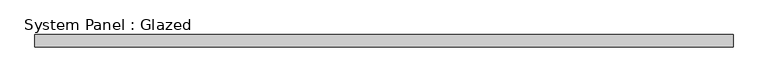
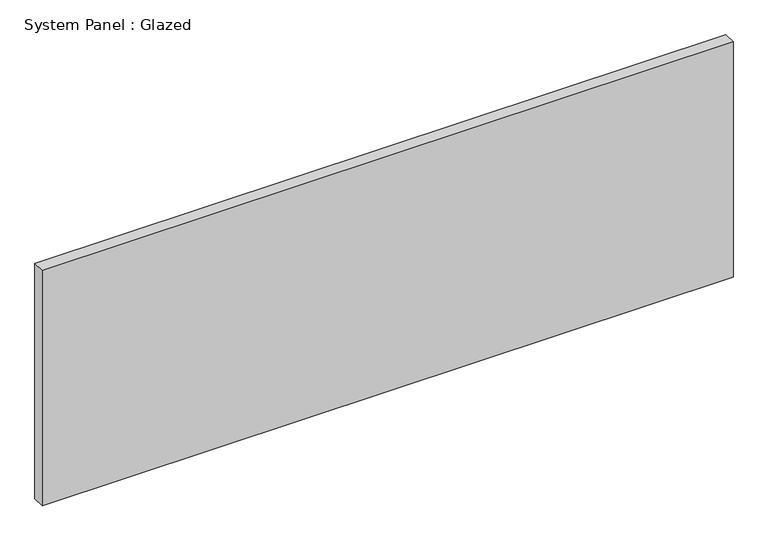
"""IFC4 building model written with IfcOpenShell, lengths in millimetres: plate geometry, System Panel : Glazed."""

from ifc_helpers import new_model, si_unit, origin, origin_with_axes, place, context, project, spatial, polyline, outline, extrude, source, transform, mapped, element, save


def system_panel_glazed_cd562e5d(model_context):
    return source(origin(), model_context, "Body", "SweptSolid", [
        extrude(outline(polyline([(714.375, -44.45), (-714.375, -44.45), (-714.375, -19.05), (714.375, -19.05), (714.375, -44.45)])), origin_with_axes(), (0.0, 0.0, 1.0), 514.35),
    ])


if __name__ == "__main__":
    model = new_model("IFC4")
    model_context = context("Model", 3, world=origin())
    ifc_project = project(units=[si_unit("LENGTHUNIT", "METRE", prefix="MILLI")], contexts=[model_context])
    site = spatial("IfcSite", under=ifc_project)
    building = spatial("IfcBuilding", under=site)
    placement = place(None, origin())
    system_panel_glazed_shape = system_panel_glazed_cd562e5d(model_context)
    element("IfcPlate", 1, ObjectType="System Panel : Glazed", at=placement, inside=building, context=model_context, shape_type="MappedRepresentation", body=[
        mapped(system_panel_glazed_shape, transform((0.0, 0.0, 0.0), x_axis=(1.0, 0.0, 0.0), y_axis=(0.0, 1.0, 0.0), z_axis=(0.0, 0.0, 1.0))),
    ])
    save(model, "model.ifc")

# Revit data of these elements
# Type "System Panel : Glazed"
#   Construction Type Id = "GSP4R"
#   Analytic Construction = "1/8 in Pilkington single glazing"
#   Visual Light Transmittance = 0.9
#   Solar Heat Gain Coefficient = 0.86
#   Heat Transfer Coefficient (U) = 1.18115 BTU/(h·ft²·°F)
# Element 1 (IfcPlate, "System Panel : Glazed")
#   Materials on its faces: "Glass"
# Materials
#   "Glass": class "Glass", colour RGB 0 128 192, transparency 0.75, Description = "Soda Lime Glass", Cost = 0
